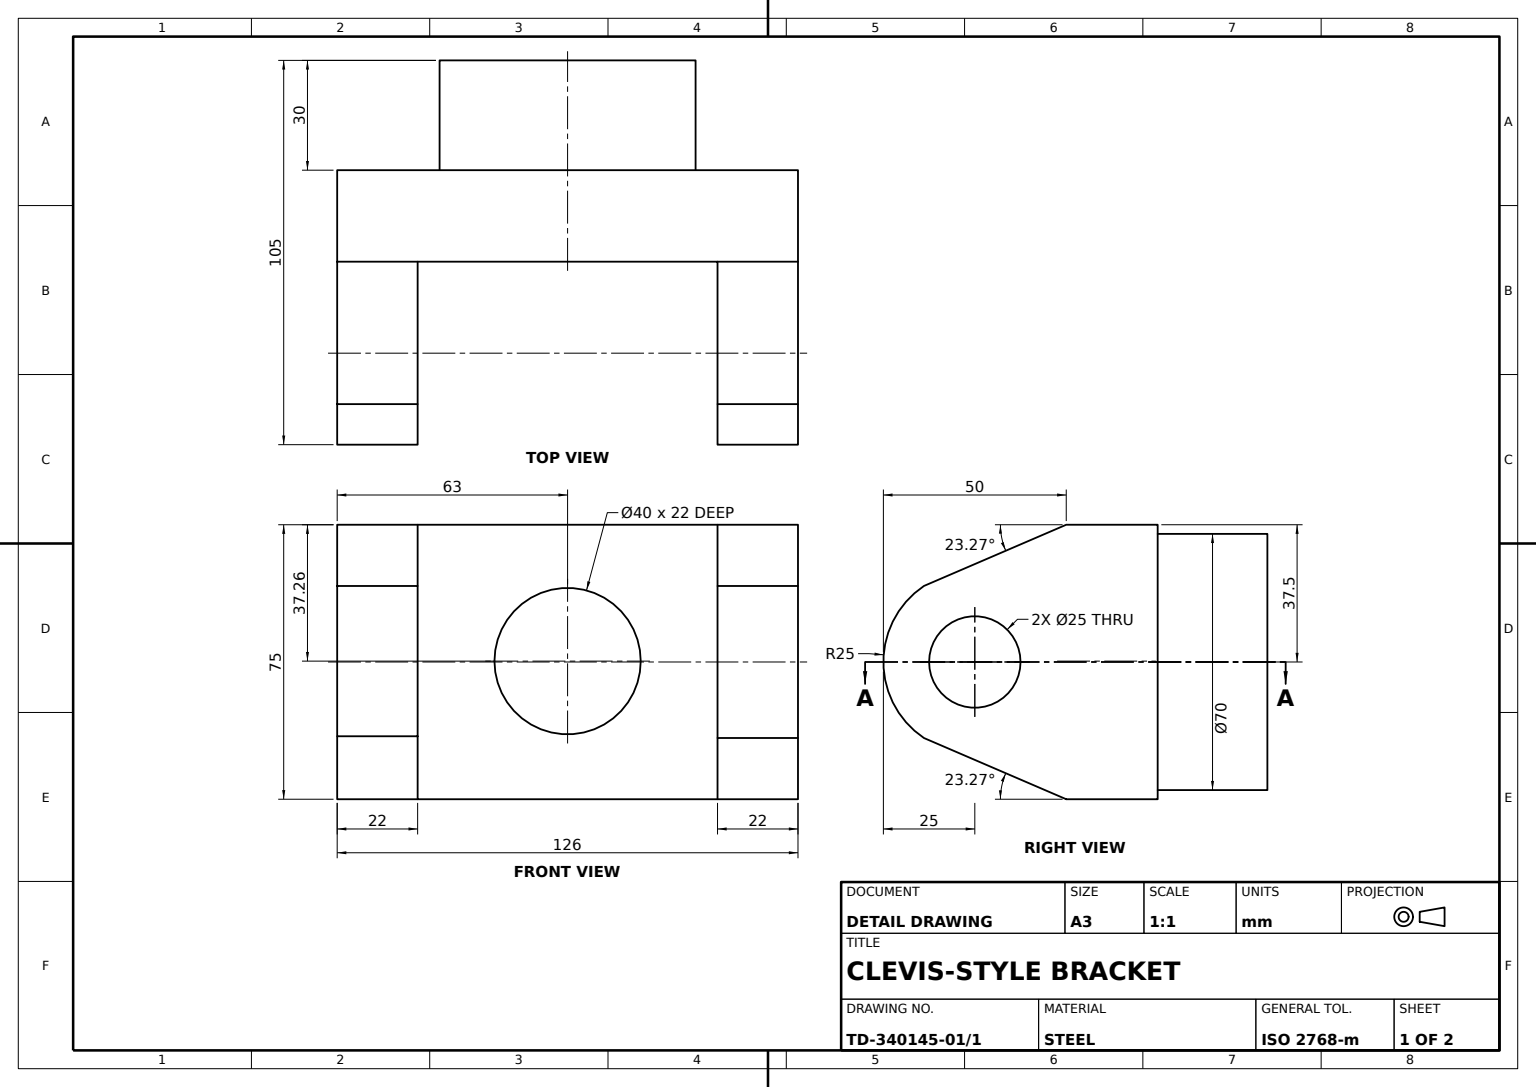
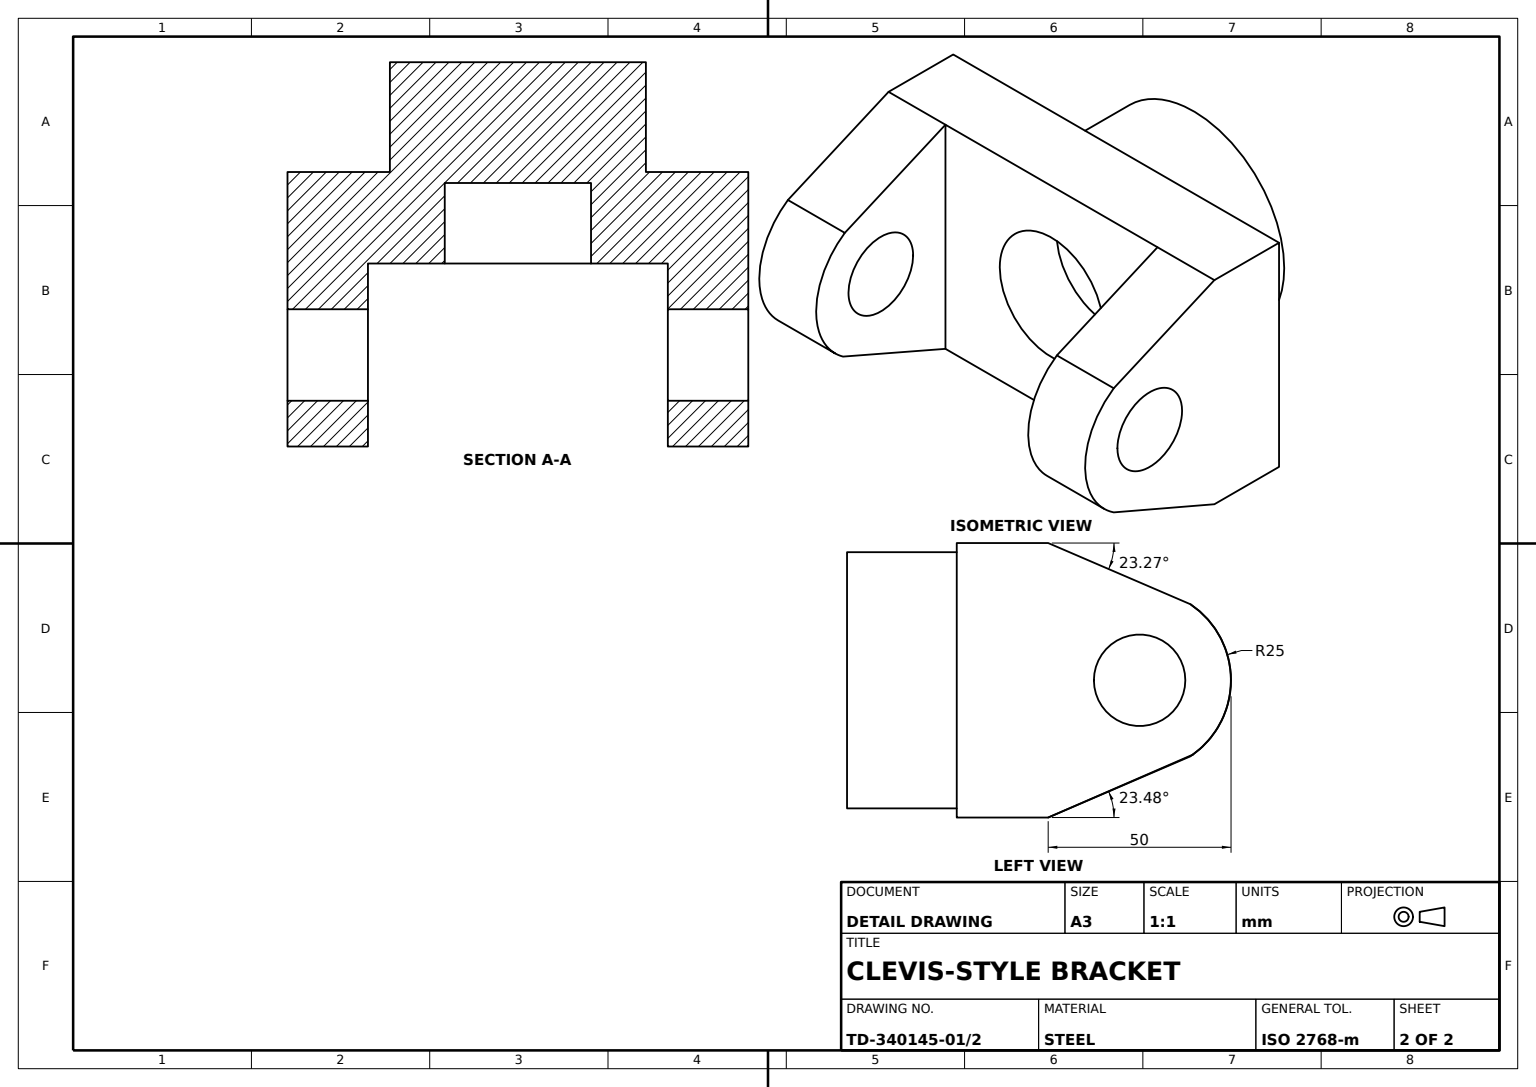
SolidWorks part; units mm, degrees
material "Plain Carbon Steel"
ref_plane "Front Plane" through (0, 0, 0) normal (0, 0, 1) x (1, 0, 0)
ref_plane "Top Plane" through (0, 0, 0) normal (0, 1, 0) x (1, 0, 0)
ref_plane "Right Plane" through (0, 0, 0) normal (1, 0, 0) x (0, 0, -1)
sketch "Base Plate Sketch" plane through (0, 0, 0) normal (0, 0, 1) x (1, 0, 0)
  line L0 (0, 0) -> (126, 0)
  line L1 (126, 0) -> (126, 75)
  line L2 (126, 75) -> (0, 75)
  line L3 (0, 75) -> (0, 0)
  dimension "D1" = 126
  dimension "D2" = 75
extrude "Base Plate" add sketch "Base Plate Sketch" along normal blind 25
sketch "Lug 1 Sketch" plane through (126, 0, 0) normal (1, 0, 0) x (0, 0, -1)
  line L0 (-25, 75) -> (-25, 0)
  line L1 (0, 0) -> (0, 75) construction
  line L2 (-25, 75) -> (-63.919, 58.2668)
  line L3 (-25, 0) -> (-63.919, 16.7332)
  arc A0 (-63.919, 58.2668) -> (-63.919, 16.7332) centre (-50, 37.5) ccw
  dimension "D1" = 50
  dimension "D2" = 25
  dimension "D3" = 63.919
extrude "Lug 1" add sketch "Lug 1 Sketch" against normal blind 22
sketch "Lug 2 Sketch" plane through (0, 0, 0) normal (-1, 0, 0) x (0, 0, 1)
  line L0 (25, 75) -> (25, 0)
  line L1 (0, 75) -> (0, 0) construction
  line L2 (25, 75) -> (63.919, 58.2668)
  line L3 (25, 75) -> (63.919, 58.2668) construction
  line L4 (25, 0) -> (64.5998, 17.206)
  arc A0 (64.5998, 17.206) -> (63.919, 58.2668) centre (50, 37.5) ccw
  dimension "D1" = 50
  dimension "D2" = 25
  dimension "D3" = 63.919
  dimension "D4" = 64.5998
extrude "Lug 2" add sketch "Lug 2 Sketch" against normal blind 22
sketch "Centre Bore Sketch" plane through (0, 0, 25) normal (0, 0, 1) x (1, 0, 0)
  line L0 (22, 75) -> (22, 0) construction
  line L1 (104, 75) -> (22, 75) construction
  circle A0 centre (63, 37.7364) radius 20
  dimension "D1" = 40
  dimension "D2" = 40
  dimension "D3" = 41
  dimension "D4" = 37.2636
extrude "Centre Bore Ø40" cut sketch "Centre Bore Sketch" against normal blind 22
sketch "Rear Boss Sketch" plane through (0, 0, 0) normal (0, 0, -1) x (-1, 0, 0)
  line L0 (0, 75) -> (0, 0) construction
  line L1 (-126, 75) -> (0, 75) construction
  circle A1 centre (-63, 37.5) radius 35
  dimension "D1" = 70
  dimension "D2" = 70
  dimension "D3" = 63
  dimension "D4" = 37.5
extrude "Rear Boss Ø70" add sketch "Rear Boss Sketch" along normal blind 30
sketch "Lug Hole 1 Sketch" plane through (0, 0, 0) normal (-1, 0, 0) x (0, 0, 1)
  line L0 (0, 75) -> (0, 0) construction
  line L1 (25, 0) -> (0, 0) construction
  circle A0 centre (50, 37.5) radius 12.5
  dimension "D1" = 25
  dimension "D2" = 25
  dimension "D3" = 50
  dimension "D4" = 37.5
extrude "Lug Hole 1 Ø25" cut sketch "Lug Hole 1 Sketch" against normal blind 22
sketch "Lug Hole 2 Sketch" plane through (126, 0, 0) normal (1, 0, 0) x (0, 0, -1)
  circle A0 centre (-50, 37.5) radius 12.5
  dimension "D1" = 25
  dimension "D2" = 25
extrude "Lug Hole 2 Ø25" cut sketch "Lug Hole 2 Sketch" against normal blind 22
